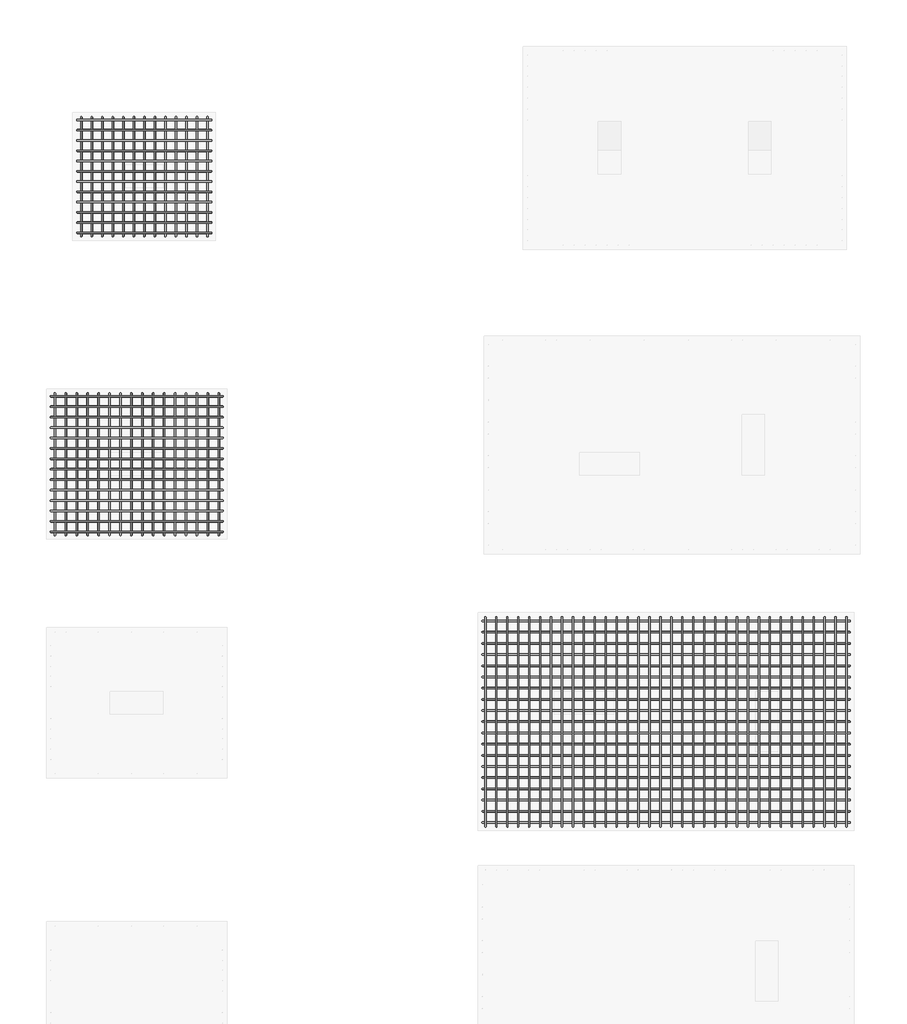
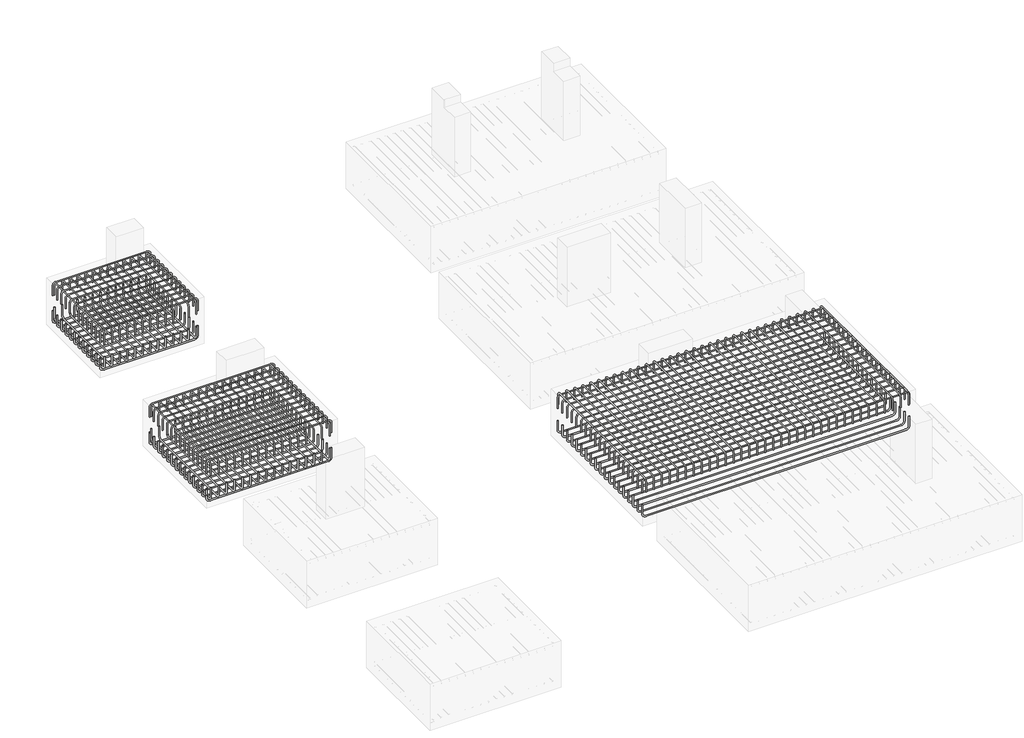
# One storey, part 11 of 21: 11 reinforcing bars.
"""IFC4 building model written with IfcOpenShell, lengths in millimetres."""

from ifc_helpers import new_model, si_unit, point, frame, origin, place, context, project, spatial, polyline, circle_curve, trimmed, segment, composite_curve, source, transform, mapped, element, save
from ifc_brep_helpers import swept_disk

model = new_model("IFC4")

# Units and contexts
model_context = context("Model", 3, world=origin())
ifc_project = project(units=[si_unit("LENGTHUNIT", "METRE", prefix="MILLI")], contexts=[model_context])

# Site, building, storey
site = spatial("IfcSite", under=ifc_project)
building = spatial("IfcBuilding", under=site)
storey = spatial("IfcBuildingStorey", under=building, Elevation=-1100.0)

# Reinforcing bars
placement = place(None, origin())
reinforcing_bar_shape = source(origin(), model_context, "Body", "SolidModel", [
    swept_disk(composite_curve([segment(polyline([(-23210.8326863, 15207.9216575, -1700.0), (-23210.8326863, 15207.9216575, -1882.5)]), True, "CONTINUOUS"), segment(trimmed(circle_curve(frame((-23268.3326863, 15207.9216575, -1882.5), z_axis=(0.0, 1.0, 0.0), x_axis=(57.5, 0.0, 0.0)), 57.5), [point((-23210.8326863, 15207.9216575, -1882.5))], [point((-23268.3326863, 15207.9216575, -1940.0))], True, "CARTESIAN"), True, "CONTINUOUS"), segment(polyline([(-23268.3326863, 15207.9216575, -1940.0), (-24933.3326863, 15207.9216575, -1940.0)]), True, "CONTINUOUS"), segment(trimmed(circle_curve(frame((-24933.3326863, 15207.9216575, -1882.5), z_axis=(0.0, 1.0, 0.0), x_axis=(0.0, 0.0, -57.5)), 57.5), [point((-24933.3326863, 15207.9216575, -1940.0))], [point((-24990.8326863, 15207.9216575, -1882.5))], True, "CARTESIAN"), True, "CONTINUOUS"), segment(polyline([(-24990.8326863, 15207.9216575, -1882.5), (-24990.8326863, 15207.9216575, -1700.0)]), True, "CONTINUOUS")], self_intersect=False), 10.0),
])
element("IfcReinforcingBar", 1, at=placement, inside=storey, context=model_context, shape_type="MappedRepresentation", body=[
    mapped(reinforcing_bar_shape, transform((0.0, 0.0, 0.0), x_axis=(1.0, 0.0, 0.0), y_axis=(0.0, 1.0, 0.0), z_axis=(0.0, 0.0, 1.0))),
    mapped(reinforcing_bar_shape, transform((0.0, -136.5188719, 0.0), x_axis=(1.0, 0.0, 0.0), y_axis=(0.0, 1.0, 0.0), z_axis=(0.0, 0.0, 1.0))),
    mapped(reinforcing_bar_shape, transform((0.0, -273.0377439, 0.0), x_axis=(1.0, 0.0, 0.0), y_axis=(0.0, 1.0, 0.0), z_axis=(0.0, 0.0, 1.0))),
    mapped(reinforcing_bar_shape, transform((0.0, -409.5566158, 0.0), x_axis=(1.0, 0.0, 0.0), y_axis=(0.0, 1.0, 0.0), z_axis=(0.0, 0.0, 1.0))),
    mapped(reinforcing_bar_shape, transform((0.0, -546.0754878, 0.0), x_axis=(1.0, 0.0, 0.0), y_axis=(0.0, 1.0, 0.0), z_axis=(0.0, 0.0, 1.0))),
    mapped(reinforcing_bar_shape, transform((0.0, -682.5943597, 0.0), x_axis=(1.0, 0.0, 0.0), y_axis=(0.0, 1.0, 0.0), z_axis=(0.0, 0.0, 1.0))),
    mapped(reinforcing_bar_shape, transform((0.0, -819.1132316, 0.0), x_axis=(1.0, 0.0, 0.0), y_axis=(0.0, 1.0, 0.0), z_axis=(0.0, 0.0, 1.0))),
    mapped(reinforcing_bar_shape, transform((0.0, -955.6321036, 0.0), x_axis=(1.0, 0.0, 0.0), y_axis=(0.0, 1.0, 0.0), z_axis=(0.0, 0.0, 1.0))),
    mapped(reinforcing_bar_shape, transform((0.0, -1092.1509755, 0.0), x_axis=(1.0, 0.0, 0.0), y_axis=(0.0, 1.0, 0.0), z_axis=(0.0, 0.0, 1.0))),
    mapped(reinforcing_bar_shape, transform((0.0, -1228.6698475, 0.0), x_axis=(1.0, 0.0, 0.0), y_axis=(0.0, 1.0, 0.0), z_axis=(0.0, 0.0, 1.0))),
    mapped(reinforcing_bar_shape, transform((0.0, -1365.1887194, 0.0), x_axis=(1.0, 0.0, 0.0), y_axis=(0.0, 1.0, 0.0), z_axis=(0.0, 0.0, 1.0))),
    mapped(reinforcing_bar_shape, transform((0.0, -1501.7075913, 0.0), x_axis=(1.0, 0.0, 0.0), y_axis=(0.0, 1.0, 0.0), z_axis=(0.0, 0.0, 1.0))),
])
reinforcing_bar_2_shape = source(origin(), model_context, "Body", "SolidModel", [
    swept_disk(composite_curve([segment(polyline([(-24992.8826863, 15207.9216575, -1400.0), (-24992.8826863, 15207.9216575, -1213.4)]), True, "CONTINUOUS"), segment(trimmed(circle_curve(frame((-24937.4326863, 15207.9216575, -1213.4), z_axis=(0.0, 1.0, 0.0), x_axis=(-55.45000000000073, 0.0, 0.0)), 55.45), [point((-24992.8826863, 15207.9216575, -1213.4))], [point((-24937.4326863, 15207.9216575, -1157.95))], True, "CARTESIAN"), True, "CONTINUOUS"), segment(polyline([(-24937.4326863, 15207.9216575, -1157.95), (-23264.2326863, 15207.9216575, -1157.95)]), True, "CONTINUOUS"), segment(trimmed(circle_curve(frame((-23264.2326863, 15207.9216575, -1213.4), z_axis=(0.0, 1.0, 0.0), x_axis=(0.0, 0.0, 55.450000000000045)), 55.45), [point((-23264.2326863, 15207.9216575, -1157.95))], [point((-23208.7826863, 15207.9216575, -1213.4))], True, "CARTESIAN"), True, "CONTINUOUS"), segment(polyline([(-23208.7826863, 15207.9216575, -1213.4), (-23208.7826863, 15207.9216575, -1400.0)]), True, "CONTINUOUS")], self_intersect=False), 7.95),
])
element("IfcReinforcingBar", 2, at=placement, inside=storey, context=model_context, shape_type="MappedRepresentation", body=[
    mapped(reinforcing_bar_2_shape, transform((0.0, 0.0, 0.0), x_axis=(1.0, 0.0, 0.0), y_axis=(0.0, 1.0, 0.0), z_axis=(0.0, 0.0, 1.0))),
    mapped(reinforcing_bar_2_shape, transform((0.0, -136.5188719, 0.0), x_axis=(1.0, 0.0, 0.0), y_axis=(0.0, 1.0, 0.0), z_axis=(0.0, 0.0, 1.0))),
    mapped(reinforcing_bar_2_shape, transform((0.0, -273.0377439, 0.0), x_axis=(1.0, 0.0, 0.0), y_axis=(0.0, 1.0, 0.0), z_axis=(0.0, 0.0, 1.0))),
    mapped(reinforcing_bar_2_shape, transform((0.0, -409.5566158, 0.0), x_axis=(1.0, 0.0, 0.0), y_axis=(0.0, 1.0, 0.0), z_axis=(0.0, 0.0, 1.0))),
    mapped(reinforcing_bar_2_shape, transform((0.0, -546.0754878, 0.0), x_axis=(1.0, 0.0, 0.0), y_axis=(0.0, 1.0, 0.0), z_axis=(0.0, 0.0, 1.0))),
    mapped(reinforcing_bar_2_shape, transform((0.0, -682.5943597, 0.0), x_axis=(1.0, 0.0, 0.0), y_axis=(0.0, 1.0, 0.0), z_axis=(0.0, 0.0, 1.0))),
    mapped(reinforcing_bar_2_shape, transform((0.0, -819.1132316, 0.0), x_axis=(1.0, 0.0, 0.0), y_axis=(0.0, 1.0, 0.0), z_axis=(0.0, 0.0, 1.0))),
    mapped(reinforcing_bar_2_shape, transform((0.0, -955.6321036, 0.0), x_axis=(1.0, 0.0, 0.0), y_axis=(0.0, 1.0, 0.0), z_axis=(0.0, 0.0, 1.0))),
    mapped(reinforcing_bar_2_shape, transform((0.0, -1092.1509755, 0.0), x_axis=(1.0, 0.0, 0.0), y_axis=(0.0, 1.0, 0.0), z_axis=(0.0, 0.0, 1.0))),
    mapped(reinforcing_bar_2_shape, transform((0.0, -1228.6698475, 0.0), x_axis=(1.0, 0.0, 0.0), y_axis=(0.0, 1.0, 0.0), z_axis=(0.0, 0.0, 1.0))),
    mapped(reinforcing_bar_2_shape, transform((0.0, -1365.1887194, 0.0), x_axis=(1.0, 0.0, 0.0), y_axis=(0.0, 1.0, 0.0), z_axis=(0.0, 0.0, 1.0))),
    mapped(reinforcing_bar_2_shape, transform((0.0, -1501.7075913, 0.0), x_axis=(1.0, 0.0, 0.0), y_axis=(0.0, 1.0, 0.0), z_axis=(0.0, 0.0, 1.0))),
])
reinforcing_bar_3_shape = source(origin(), model_context, "Body", "SolidModel", [
    swept_disk(composite_curve([segment(polyline([(-23260.6168504, 15246.2204288, -1428.1111113), (-23260.6168504, 15246.2204288, -1241.5111113)]), True, "CONTINUOUS"), segment(trimmed(circle_curve(frame((-23260.6168504, 15190.7704288, -1241.5111113), z_axis=(1.0, 0.0, 0.0), x_axis=(0.0, 55.44999999999891, 0.0)), 55.45), [point((-23260.6168504, 15246.2204288, -1241.5111113))], [point((-23260.6168504, 15190.7704288, -1186.0611113))], True, "CARTESIAN"), True, "CONTINUOUS"), segment(polyline([(-23260.6168504, 15190.7704288, -1186.0611113), (-23260.6168504, 13717.5704288, -1186.0611113)]), True, "CONTINUOUS"), segment(trimmed(circle_curve(frame((-23260.6168504, 13717.5704288, -1241.5111113), z_axis=(1.0, 0.0, 0.0), x_axis=(0.0, 0.0, 55.450000000000045)), 55.45), [point((-23260.6168504, 13717.5704288, -1186.0611113))], [point((-23260.6168504, 13662.1204288, -1241.5111113))], True, "CARTESIAN"), True, "CONTINUOUS"), segment(polyline([(-23260.6168504, 13662.1204288, -1241.5111113), (-23260.6168504, 13662.1204288, -1428.1111113)]), True, "CONTINUOUS")], self_intersect=False), 7.95),
])
element("IfcReinforcingBar", 3, at=placement, inside=storey, context=model_context, shape_type="MappedRepresentation", body=[
    mapped(reinforcing_bar_3_shape, transform((0.0, 0.0, 0.0), x_axis=(1.0, 0.0, 0.0), y_axis=(0.0, 1.0, 0.0), z_axis=(0.0, 0.0, 1.0))),
    mapped(reinforcing_bar_3_shape, transform((-139.8994495, 0.0, 0.0), x_axis=(1.0, 0.0, 0.0), y_axis=(0.0, 1.0, 0.0), z_axis=(0.0, 0.0, 1.0))),
    mapped(reinforcing_bar_3_shape, transform((-279.7988989, 0.0, 0.0), x_axis=(1.0, 0.0, 0.0), y_axis=(0.0, 1.0, 0.0), z_axis=(0.0, 0.0, 1.0))),
    mapped(reinforcing_bar_3_shape, transform((-419.6983484, 0.0, 0.0), x_axis=(1.0, 0.0, 0.0), y_axis=(0.0, 1.0, 0.0), z_axis=(0.0, 0.0, 1.0))),
    mapped(reinforcing_bar_3_shape, transform((-559.5977978, 0.0, 0.0), x_axis=(1.0, 0.0, 0.0), y_axis=(0.0, 1.0, 0.0), z_axis=(0.0, 0.0, 1.0))),
    mapped(reinforcing_bar_3_shape, transform((-699.4972473, 0.0, 0.0), x_axis=(1.0, 0.0, 0.0), y_axis=(0.0, 1.0, 0.0), z_axis=(0.0, 0.0, 1.0))),
    mapped(reinforcing_bar_3_shape, transform((-839.3966967, 0.0, 0.0), x_axis=(1.0, 0.0, 0.0), y_axis=(0.0, 1.0, 0.0), z_axis=(0.0, 0.0, 1.0))),
    mapped(reinforcing_bar_3_shape, transform((-979.2961462, 0.0, 0.0), x_axis=(1.0, 0.0, 0.0), y_axis=(0.0, 1.0, 0.0), z_axis=(0.0, 0.0, 1.0))),
    mapped(reinforcing_bar_3_shape, transform((-1119.1955956, 0.0, 0.0), x_axis=(1.0, 0.0, 0.0), y_axis=(0.0, 1.0, 0.0), z_axis=(0.0, 0.0, 1.0))),
    mapped(reinforcing_bar_3_shape, transform((-1259.0950451, 0.0, 0.0), x_axis=(1.0, 0.0, 0.0), y_axis=(0.0, 1.0, 0.0), z_axis=(0.0, 0.0, 1.0))),
    mapped(reinforcing_bar_3_shape, transform((-1398.9944945, 0.0, 0.0), x_axis=(1.0, 0.0, 0.0), y_axis=(0.0, 1.0, 0.0), z_axis=(0.0, 0.0, 1.0))),
    mapped(reinforcing_bar_3_shape, transform((-1538.893944, 0.0, 0.0), x_axis=(1.0, 0.0, 0.0), y_axis=(0.0, 1.0, 0.0), z_axis=(0.0, 0.0, 1.0))),
    mapped(reinforcing_bar_3_shape, transform((-1678.7933934, 0.0, 0.0), x_axis=(1.0, 0.0, 0.0), y_axis=(0.0, 1.0, 0.0), z_axis=(0.0, 0.0, 1.0))),
])
reinforcing_bar_4_shape = source(origin(), model_context, "Body", "SolidModel", [
    swept_disk(composite_curve([segment(polyline([(-24939.4102438, 15244.1704288, -1669.8442859), (-24939.4102438, 15244.1704288, -1852.3442859)]), True, "CONTINUOUS"), segment(trimmed(circle_curve(frame((-24939.4102438, 15186.6704288, -1852.3442859), z_axis=(-1.0, 0.0, 0.0), x_axis=(0.0, 57.5, 0.0)), 57.5), [point((-24939.4102438, 15244.1704288, -1852.3442859))], [point((-24939.4102438, 15186.6704288, -1909.8442859))], True, "CARTESIAN"), True, "CONTINUOUS"), segment(polyline([(-24939.4102438, 15186.6704288, -1909.8442859), (-24939.4102438, 13721.6704288, -1909.8442859)]), True, "CONTINUOUS"), segment(trimmed(circle_curve(frame((-24939.4102438, 13721.6704288, -1852.3442859), z_axis=(-1.0, 0.0, 0.0), x_axis=(0.0, 0.0, -57.5)), 57.5), [point((-24939.4102438, 13721.6704288, -1909.8442859))], [point((-24939.4102438, 13664.1704288, -1852.3442859))], True, "CARTESIAN"), True, "CONTINUOUS"), segment(polyline([(-24939.4102438, 13664.1704288, -1852.3442859), (-24939.4102438, 13664.1704288, -1669.8442859)]), True, "CONTINUOUS")], self_intersect=False), 10.0),
])
element("IfcReinforcingBar", 4, at=placement, inside=storey, context=model_context, shape_type="MappedRepresentation", body=[
    mapped(reinforcing_bar_4_shape, transform((0.0, 0.0, 0.0), x_axis=(1.0, 0.0, 0.0), y_axis=(0.0, 1.0, 0.0), z_axis=(0.0, 0.0, 1.0))),
    mapped(reinforcing_bar_4_shape, transform((139.8994495, 0.0, 0.0), x_axis=(1.0, 0.0, 0.0), y_axis=(0.0, 1.0, 0.0), z_axis=(0.0, 0.0, 1.0))),
    mapped(reinforcing_bar_4_shape, transform((279.7988989, 0.0, 0.0), x_axis=(1.0, 0.0, 0.0), y_axis=(0.0, 1.0, 0.0), z_axis=(0.0, 0.0, 1.0))),
    mapped(reinforcing_bar_4_shape, transform((419.6983484, 0.0, 0.0), x_axis=(1.0, 0.0, 0.0), y_axis=(0.0, 1.0, 0.0), z_axis=(0.0, 0.0, 1.0))),
    mapped(reinforcing_bar_4_shape, transform((559.5977978, 0.0, 0.0), x_axis=(1.0, 0.0, 0.0), y_axis=(0.0, 1.0, 0.0), z_axis=(0.0, 0.0, 1.0))),
    mapped(reinforcing_bar_4_shape, transform((699.4972473, 0.0, 0.0), x_axis=(1.0, 0.0, 0.0), y_axis=(0.0, 1.0, 0.0), z_axis=(0.0, 0.0, 1.0))),
    mapped(reinforcing_bar_4_shape, transform((839.3966967, 0.0, 0.0), x_axis=(1.0, 0.0, 0.0), y_axis=(0.0, 1.0, 0.0), z_axis=(0.0, 0.0, 1.0))),
    mapped(reinforcing_bar_4_shape, transform((979.2961462, 0.0, 0.0), x_axis=(1.0, 0.0, 0.0), y_axis=(0.0, 1.0, 0.0), z_axis=(0.0, 0.0, 1.0))),
    mapped(reinforcing_bar_4_shape, transform((1119.1955956, 0.0, 0.0), x_axis=(1.0, 0.0, 0.0), y_axis=(0.0, 1.0, 0.0), z_axis=(0.0, 0.0, 1.0))),
    mapped(reinforcing_bar_4_shape, transform((1259.0950451, 0.0, 0.0), x_axis=(1.0, 0.0, 0.0), y_axis=(0.0, 1.0, 0.0), z_axis=(0.0, 0.0, 1.0))),
    mapped(reinforcing_bar_4_shape, transform((1398.9944945, 0.0, 0.0), x_axis=(1.0, 0.0, 0.0), y_axis=(0.0, 1.0, 0.0), z_axis=(0.0, 0.0, 1.0))),
    mapped(reinforcing_bar_4_shape, transform((1538.893944, 0.0, 0.0), x_axis=(1.0, 0.0, 0.0), y_axis=(0.0, 1.0, 0.0), z_axis=(0.0, 0.0, 1.0))),
    mapped(reinforcing_bar_4_shape, transform((1678.7933934, 0.0, 0.0), x_axis=(1.0, 0.0, 0.0), y_axis=(0.0, 1.0, 0.0), z_axis=(0.0, 0.0, 1.0))),
])
reinforcing_bar_5_shape = source(origin(), model_context, "Body", "SolidModel", [
    swept_disk(composite_curve([segment(polyline([(-23061.1351198, 11532.9767109, -1700.0), (-23061.1351198, 11532.9767109, -1882.5)]), True, "CONTINUOUS"), segment(trimmed(circle_curve(frame((-23118.6351198, 11532.9767109, -1882.5), z_axis=(0.0, 1.0, 0.0), x_axis=(57.5, 0.0, 0.0)), 57.5), [point((-23061.1351198, 11532.9767109, -1882.5))], [point((-23118.6351198, 11532.9767109, -1940.0))], True, "CARTESIAN"), True, "CONTINUOUS"), segment(polyline([(-23118.6351198, 11532.9767109, -1940.0), (-25283.6351198, 11532.9767109, -1940.0)]), True, "CONTINUOUS"), segment(trimmed(circle_curve(frame((-25283.6351198, 11532.9767109, -1882.5), z_axis=(0.0, 1.0, 0.0), x_axis=(0.0, 0.0, -57.5)), 57.5), [point((-25283.6351198, 11532.9767109, -1940.0))], [point((-25341.1351198, 11532.9767109, -1882.5))], True, "CARTESIAN"), True, "CONTINUOUS"), segment(polyline([(-25341.1351198, 11532.9767109, -1882.5), (-25341.1351198, 11532.9767109, -1700.0)]), True, "CONTINUOUS")], self_intersect=False), 10.0),
])
element("IfcReinforcingBar", 5, at=placement, inside=storey, context=model_context, shape_type="MappedRepresentation", body=[
    mapped(reinforcing_bar_5_shape, transform((0.0, 0.0, 0.0), x_axis=(1.0, 0.0, 0.0), y_axis=(0.0, 1.0, 0.0), z_axis=(0.0, 0.0, 1.0))),
    mapped(reinforcing_bar_5_shape, transform((0.0, -138.5928916, 0.0), x_axis=(1.0, 0.0, 0.0), y_axis=(0.0, 1.0, 0.0), z_axis=(0.0, 0.0, 1.0))),
    mapped(reinforcing_bar_5_shape, transform((0.0, -277.1857833, 0.0), x_axis=(1.0, 0.0, 0.0), y_axis=(0.0, 1.0, 0.0), z_axis=(0.0, 0.0, 1.0))),
    mapped(reinforcing_bar_5_shape, transform((0.0, -415.7786749, 0.0), x_axis=(1.0, 0.0, 0.0), y_axis=(0.0, 1.0, 0.0), z_axis=(0.0, 0.0, 1.0))),
    mapped(reinforcing_bar_5_shape, transform((0.0, -554.3715666, 0.0), x_axis=(1.0, 0.0, 0.0), y_axis=(0.0, 1.0, 0.0), z_axis=(0.0, 0.0, 1.0))),
    mapped(reinforcing_bar_5_shape, transform((0.0, -692.9644582, 0.0), x_axis=(1.0, 0.0, 0.0), y_axis=(0.0, 1.0, 0.0), z_axis=(0.0, 0.0, 1.0))),
    mapped(reinforcing_bar_5_shape, transform((0.0, -831.5573499, 0.0), x_axis=(1.0, 0.0, 0.0), y_axis=(0.0, 1.0, 0.0), z_axis=(0.0, 0.0, 1.0))),
    mapped(reinforcing_bar_5_shape, transform((0.0, -970.1502415, 0.0), x_axis=(1.0, 0.0, 0.0), y_axis=(0.0, 1.0, 0.0), z_axis=(0.0, 0.0, 1.0))),
    mapped(reinforcing_bar_5_shape, transform((0.0, -1108.7431331, 0.0), x_axis=(1.0, 0.0, 0.0), y_axis=(0.0, 1.0, 0.0), z_axis=(0.0, 0.0, 1.0))),
    mapped(reinforcing_bar_5_shape, transform((0.0, -1247.3360248, 0.0), x_axis=(1.0, 0.0, 0.0), y_axis=(0.0, 1.0, 0.0), z_axis=(0.0, 0.0, 1.0))),
    mapped(reinforcing_bar_5_shape, transform((0.0, -1385.9289164, 0.0), x_axis=(1.0, 0.0, 0.0), y_axis=(0.0, 1.0, 0.0), z_axis=(0.0, 0.0, 1.0))),
    mapped(reinforcing_bar_5_shape, transform((0.0, -1524.5218081, 0.0), x_axis=(1.0, 0.0, 0.0), y_axis=(0.0, 1.0, 0.0), z_axis=(0.0, 0.0, 1.0))),
    mapped(reinforcing_bar_5_shape, transform((0.0, -1663.1146997, 0.0), x_axis=(1.0, 0.0, 0.0), y_axis=(0.0, 1.0, 0.0), z_axis=(0.0, 0.0, 1.0))),
    mapped(reinforcing_bar_5_shape, transform((0.0, -1801.7075913, 0.0), x_axis=(1.0, 0.0, 0.0), y_axis=(0.0, 1.0, 0.0), z_axis=(0.0, 0.0, 1.0))),
])
reinforcing_bar_6_shape = source(origin(), model_context, "Body", "SolidModel", [
    swept_disk(composite_curve([segment(polyline([(-25343.1851198, 11532.9767109, -1400.0), (-25343.1851198, 11532.9767109, -1213.4)]), True, "CONTINUOUS"), segment(trimmed(circle_curve(frame((-25287.7351198, 11532.9767109, -1213.4), z_axis=(0.0, 1.0, 0.0), x_axis=(-55.45000000000073, 0.0, 0.0)), 55.45), [point((-25343.1851198, 11532.9767109, -1213.4))], [point((-25287.7351198, 11532.9767109, -1157.95))], True, "CARTESIAN"), True, "CONTINUOUS"), segment(polyline([(-25287.7351198, 11532.9767109, -1157.95), (-23114.5351198, 11532.9767109, -1157.95)]), True, "CONTINUOUS"), segment(trimmed(circle_curve(frame((-23114.5351198, 11532.9767109, -1213.4), z_axis=(0.0, 1.0, 0.0), x_axis=(0.0, 0.0, 55.450000000000045)), 55.45), [point((-23114.5351198, 11532.9767109, -1157.95))], [point((-23059.0851198, 11532.9767109, -1213.4))], True, "CARTESIAN"), True, "CONTINUOUS"), segment(polyline([(-23059.0851198, 11532.9767109, -1213.4), (-23059.0851198, 11532.9767109, -1400.0)]), True, "CONTINUOUS")], self_intersect=False), 7.95),
])
element("IfcReinforcingBar", 6, at=placement, inside=storey, context=model_context, shape_type="MappedRepresentation", body=[
    mapped(reinforcing_bar_6_shape, transform((0.0, 0.0, 0.0), x_axis=(1.0, 0.0, 0.0), y_axis=(0.0, 1.0, 0.0), z_axis=(0.0, 0.0, 1.0))),
    mapped(reinforcing_bar_6_shape, transform((0.0, -138.5928916, 0.0), x_axis=(1.0, 0.0, 0.0), y_axis=(0.0, 1.0, 0.0), z_axis=(0.0, 0.0, 1.0))),
    mapped(reinforcing_bar_6_shape, transform((0.0, -277.1857833, 0.0), x_axis=(1.0, 0.0, 0.0), y_axis=(0.0, 1.0, 0.0), z_axis=(0.0, 0.0, 1.0))),
    mapped(reinforcing_bar_6_shape, transform((0.0, -415.7786749, 0.0), x_axis=(1.0, 0.0, 0.0), y_axis=(0.0, 1.0, 0.0), z_axis=(0.0, 0.0, 1.0))),
    mapped(reinforcing_bar_6_shape, transform((0.0, -554.3715666, 0.0), x_axis=(1.0, 0.0, 0.0), y_axis=(0.0, 1.0, 0.0), z_axis=(0.0, 0.0, 1.0))),
    mapped(reinforcing_bar_6_shape, transform((0.0, -692.9644582, 0.0), x_axis=(1.0, 0.0, 0.0), y_axis=(0.0, 1.0, 0.0), z_axis=(0.0, 0.0, 1.0))),
    mapped(reinforcing_bar_6_shape, transform((0.0, -831.5573499, 0.0), x_axis=(1.0, 0.0, 0.0), y_axis=(0.0, 1.0, 0.0), z_axis=(0.0, 0.0, 1.0))),
    mapped(reinforcing_bar_6_shape, transform((0.0, -970.1502415, 0.0), x_axis=(1.0, 0.0, 0.0), y_axis=(0.0, 1.0, 0.0), z_axis=(0.0, 0.0, 1.0))),
    mapped(reinforcing_bar_6_shape, transform((0.0, -1108.7431331, 0.0), x_axis=(1.0, 0.0, 0.0), y_axis=(0.0, 1.0, 0.0), z_axis=(0.0, 0.0, 1.0))),
    mapped(reinforcing_bar_6_shape, transform((0.0, -1247.3360248, 0.0), x_axis=(1.0, 0.0, 0.0), y_axis=(0.0, 1.0, 0.0), z_axis=(0.0, 0.0, 1.0))),
    mapped(reinforcing_bar_6_shape, transform((0.0, -1385.9289164, 0.0), x_axis=(1.0, 0.0, 0.0), y_axis=(0.0, 1.0, 0.0), z_axis=(0.0, 0.0, 1.0))),
    mapped(reinforcing_bar_6_shape, transform((0.0, -1524.5218081, 0.0), x_axis=(1.0, 0.0, 0.0), y_axis=(0.0, 1.0, 0.0), z_axis=(0.0, 0.0, 1.0))),
    mapped(reinforcing_bar_6_shape, transform((0.0, -1663.1146997, 0.0), x_axis=(1.0, 0.0, 0.0), y_axis=(0.0, 1.0, 0.0), z_axis=(0.0, 0.0, 1.0))),
    mapped(reinforcing_bar_6_shape, transform((0.0, -1801.7075913, 0.0), x_axis=(1.0, 0.0, 0.0), y_axis=(0.0, 1.0, 0.0), z_axis=(0.0, 0.0, 1.0))),
])
reinforcing_bar_7_shape = source(origin(), model_context, "Body", "SolidModel", [
    swept_disk(composite_curve([segment(polyline([(-23110.9192838, 11571.2754822, -1428.1111113), (-23110.9192838, 11571.2754822, -1241.5111113)]), True, "CONTINUOUS"), segment(trimmed(circle_curve(frame((-23110.9192838, 11515.8254822, -1241.5111113), z_axis=(1.0, 0.0, 0.0), x_axis=(0.0, 55.45000000000073, 0.0)), 55.45), [point((-23110.9192838, 11571.2754822, -1241.5111113))], [point((-23110.9192838, 11515.8254822, -1186.0611113))], True, "CARTESIAN"), True, "CONTINUOUS"), segment(polyline([(-23110.9192838, 11515.8254822, -1186.0611113), (-23110.9192838, 9742.6254822, -1186.0611113)]), True, "CONTINUOUS"), segment(trimmed(circle_curve(frame((-23110.9192838, 9742.6254822, -1241.5111113), z_axis=(1.0, 0.0, 0.0), x_axis=(0.0, 0.0, 55.450000000000045)), 55.45), [point((-23110.9192838, 9742.6254822, -1186.0611113))], [point((-23110.9192838, 9687.1754822, -1241.5111113))], True, "CARTESIAN"), True, "CONTINUOUS"), segment(polyline([(-23110.9192838, 9687.1754822, -1241.5111113), (-23110.9192838, 9687.1754822, -1428.1111113)]), True, "CONTINUOUS")], self_intersect=False), 7.95),
])
element("IfcReinforcingBar", 7, at=placement, inside=storey, context=model_context, shape_type="MappedRepresentation", body=[
    mapped(reinforcing_bar_7_shape, transform((0.0, 0.0, 0.0), x_axis=(1.0, 0.0, 0.0), y_axis=(0.0, 1.0, 0.0), z_axis=(0.0, 0.0, 1.0))),
    mapped(reinforcing_bar_7_shape, transform((-145.2528929, 0.0, 0.0), x_axis=(1.0, 0.0, 0.0), y_axis=(0.0, 1.0, 0.0), z_axis=(0.0, 0.0, 1.0))),
    mapped(reinforcing_bar_7_shape, transform((-290.5057858, 0.0, 0.0), x_axis=(1.0, 0.0, 0.0), y_axis=(0.0, 1.0, 0.0), z_axis=(0.0, 0.0, 1.0))),
    mapped(reinforcing_bar_7_shape, transform((-435.7586787, 0.0, 0.0), x_axis=(1.0, 0.0, 0.0), y_axis=(0.0, 1.0, 0.0), z_axis=(0.0, 0.0, 1.0))),
    mapped(reinforcing_bar_7_shape, transform((-581.0115716, 0.0, 0.0), x_axis=(1.0, 0.0, 0.0), y_axis=(0.0, 1.0, 0.0), z_axis=(0.0, 0.0, 1.0))),
    mapped(reinforcing_bar_7_shape, transform((-726.2644645, 0.0, 0.0), x_axis=(1.0, 0.0, 0.0), y_axis=(0.0, 1.0, 0.0), z_axis=(0.0, 0.0, 1.0))),
    mapped(reinforcing_bar_7_shape, transform((-871.5173574, 0.0, 0.0), x_axis=(1.0, 0.0, 0.0), y_axis=(0.0, 1.0, 0.0), z_axis=(0.0, 0.0, 1.0))),
    mapped(reinforcing_bar_7_shape, transform((-1016.7702503, 0.0, 0.0), x_axis=(1.0, 0.0, 0.0), y_axis=(0.0, 1.0, 0.0), z_axis=(0.0, 0.0, 1.0))),
    mapped(reinforcing_bar_7_shape, transform((-1162.0231432, 0.0, 0.0), x_axis=(1.0, 0.0, 0.0), y_axis=(0.0, 1.0, 0.0), z_axis=(0.0, 0.0, 1.0))),
    mapped(reinforcing_bar_7_shape, transform((-1307.276036, 0.0, 0.0), x_axis=(1.0, 0.0, 0.0), y_axis=(0.0, 1.0, 0.0), z_axis=(0.0, 0.0, 1.0))),
    mapped(reinforcing_bar_7_shape, transform((-1452.5289289, 0.0, 0.0), x_axis=(1.0, 0.0, 0.0), y_axis=(0.0, 1.0, 0.0), z_axis=(0.0, 0.0, 1.0))),
    mapped(reinforcing_bar_7_shape, transform((-1597.7818218, 0.0, 0.0), x_axis=(1.0, 0.0, 0.0), y_axis=(0.0, 1.0, 0.0), z_axis=(0.0, 0.0, 1.0))),
    mapped(reinforcing_bar_7_shape, transform((-1743.0347147, 0.0, 0.0), x_axis=(1.0, 0.0, 0.0), y_axis=(0.0, 1.0, 0.0), z_axis=(0.0, 0.0, 1.0))),
    mapped(reinforcing_bar_7_shape, transform((-1888.2876076, 0.0, 0.0), x_axis=(1.0, 0.0, 0.0), y_axis=(0.0, 1.0, 0.0), z_axis=(0.0, 0.0, 1.0))),
    mapped(reinforcing_bar_7_shape, transform((-2033.5405005, 0.0, 0.0), x_axis=(1.0, 0.0, 0.0), y_axis=(0.0, 1.0, 0.0), z_axis=(0.0, 0.0, 1.0))),
    mapped(reinforcing_bar_7_shape, transform((-2178.7933934, 0.0, 0.0), x_axis=(1.0, 0.0, 0.0), y_axis=(0.0, 1.0, 0.0), z_axis=(0.0, 0.0, 1.0))),
])
reinforcing_bar_8_shape = source(origin(), model_context, "Body", "SolidModel", [
    swept_disk(composite_curve([segment(polyline([(-25289.7126772, 11569.2254822, -1669.8442859), (-25289.7126772, 11569.2254822, -1852.3442859)]), True, "CONTINUOUS"), segment(trimmed(circle_curve(frame((-25289.7126772, 11511.7254822, -1852.3442859), z_axis=(-1.0, 0.0, 0.0), x_axis=(0.0, 57.5, 0.0)), 57.5), [point((-25289.7126772, 11569.2254822, -1852.3442859))], [point((-25289.7126772, 11511.7254822, -1909.8442859))], True, "CARTESIAN"), True, "CONTINUOUS"), segment(polyline([(-25289.7126772, 11511.7254822, -1909.8442859), (-25289.7126772, 9746.7254822, -1909.8442859)]), True, "CONTINUOUS"), segment(trimmed(circle_curve(frame((-25289.7126772, 9746.7254822, -1852.3442859), z_axis=(-1.0, 0.0, 0.0), x_axis=(0.0, 0.0, -57.5)), 57.5), [point((-25289.7126772, 9746.7254822, -1909.8442859))], [point((-25289.7126772, 9689.2254822, -1852.3442859))], True, "CARTESIAN"), True, "CONTINUOUS"), segment(polyline([(-25289.7126772, 9689.2254822, -1852.3442859), (-25289.7126772, 9689.2254822, -1669.8442859)]), True, "CONTINUOUS")], self_intersect=False), 10.0),
])
element("IfcReinforcingBar", 8, at=placement, inside=storey, context=model_context, shape_type="MappedRepresentation", body=[
    mapped(reinforcing_bar_8_shape, transform((0.0, 0.0, 0.0), x_axis=(1.0, 0.0, 0.0), y_axis=(0.0, 1.0, 0.0), z_axis=(0.0, 0.0, 1.0))),
    mapped(reinforcing_bar_8_shape, transform((145.2528929, 0.0, 0.0), x_axis=(1.0, 0.0, 0.0), y_axis=(0.0, 1.0, 0.0), z_axis=(0.0, 0.0, 1.0))),
    mapped(reinforcing_bar_8_shape, transform((290.5057858, 0.0, 0.0), x_axis=(1.0, 0.0, 0.0), y_axis=(0.0, 1.0, 0.0), z_axis=(0.0, 0.0, 1.0))),
    mapped(reinforcing_bar_8_shape, transform((435.7586787, 0.0, 0.0), x_axis=(1.0, 0.0, 0.0), y_axis=(0.0, 1.0, 0.0), z_axis=(0.0, 0.0, 1.0))),
    mapped(reinforcing_bar_8_shape, transform((581.0115716, 0.0, 0.0), x_axis=(1.0, 0.0, 0.0), y_axis=(0.0, 1.0, 0.0), z_axis=(0.0, 0.0, 1.0))),
    mapped(reinforcing_bar_8_shape, transform((726.2644645, 0.0, 0.0), x_axis=(1.0, 0.0, 0.0), y_axis=(0.0, 1.0, 0.0), z_axis=(0.0, 0.0, 1.0))),
    mapped(reinforcing_bar_8_shape, transform((871.5173574, 0.0, 0.0), x_axis=(1.0, 0.0, 0.0), y_axis=(0.0, 1.0, 0.0), z_axis=(0.0, 0.0, 1.0))),
    mapped(reinforcing_bar_8_shape, transform((1016.7702503, 0.0, 0.0), x_axis=(1.0, 0.0, 0.0), y_axis=(0.0, 1.0, 0.0), z_axis=(0.0, 0.0, 1.0))),
    mapped(reinforcing_bar_8_shape, transform((1162.0231432, 0.0, 0.0), x_axis=(1.0, 0.0, 0.0), y_axis=(0.0, 1.0, 0.0), z_axis=(0.0, 0.0, 1.0))),
    mapped(reinforcing_bar_8_shape, transform((1307.276036, 0.0, 0.0), x_axis=(1.0, 0.0, 0.0), y_axis=(0.0, 1.0, 0.0), z_axis=(0.0, 0.0, 1.0))),
    mapped(reinforcing_bar_8_shape, transform((1452.5289289, 0.0, 0.0), x_axis=(1.0, 0.0, 0.0), y_axis=(0.0, 1.0, 0.0), z_axis=(0.0, 0.0, 1.0))),
    mapped(reinforcing_bar_8_shape, transform((1597.7818218, 0.0, 0.0), x_axis=(1.0, 0.0, 0.0), y_axis=(0.0, 1.0, 0.0), z_axis=(0.0, 0.0, 1.0))),
    mapped(reinforcing_bar_8_shape, transform((1743.0347147, 0.0, 0.0), x_axis=(1.0, 0.0, 0.0), y_axis=(0.0, 1.0, 0.0), z_axis=(0.0, 0.0, 1.0))),
    mapped(reinforcing_bar_8_shape, transform((1888.2876076, 0.0, 0.0), x_axis=(1.0, 0.0, 0.0), y_axis=(0.0, 1.0, 0.0), z_axis=(0.0, 0.0, 1.0))),
    mapped(reinforcing_bar_8_shape, transform((2033.5405005, 0.0, 0.0), x_axis=(1.0, 0.0, 0.0), y_axis=(0.0, 1.0, 0.0), z_axis=(0.0, 0.0, 1.0))),
    mapped(reinforcing_bar_8_shape, transform((2178.7933934, 0.0, 0.0), x_axis=(1.0, 0.0, 0.0), y_axis=(0.0, 1.0, 0.0), z_axis=(0.0, 0.0, 1.0))),
])
reinforcing_bar_9_shape = source(origin(), model_context, "Body", "SolidModel", [
    swept_disk(composite_curve([segment(polyline([(-19564.5839151, 5812.1204288, -1400.0), (-19564.5839151, 5812.1204288, -1213.4)]), True, "CONTINUOUS"), segment(trimmed(circle_curve(frame((-19564.5839151, 5867.5704288, -1213.4), z_axis=(-1.0, 0.0, 0.0), x_axis=(0.0, -55.44999999999982, 0.0)), 55.45), [point((-19564.5839151, 5812.1204288, -1213.4))], [point((-19564.5839151, 5867.5704288, -1157.95))], True, "CARTESIAN"), True, "CONTINUOUS"), segment(polyline([(-19564.5839151, 5867.5704288, -1157.95), (-19564.5839151, 8540.7704288, -1157.95)]), True, "CONTINUOUS"), segment(trimmed(circle_curve(frame((-19564.5839151, 8540.7704288, -1213.4), z_axis=(-1.0, 0.0, 0.0), x_axis=(0.0, 0.0, 55.450000000000045)), 55.45), [point((-19564.5839151, 8540.7704288, -1157.95))], [point((-19564.5839151, 8596.2204288, -1213.4))], True, "CARTESIAN"), True, "CONTINUOUS"), segment(polyline([(-19564.5839151, 8596.2204288, -1213.4), (-19564.5839151, 8596.2204288, -1400.0)]), True, "CONTINUOUS")], self_intersect=False), 7.95),
])
element("IfcReinforcingBar", 9, at=placement, inside=storey, context=model_context, shape_type="MappedRepresentation", body=[
    mapped(reinforcing_bar_9_shape, transform((0.0, 0.0, 0.0), x_axis=(1.0, 0.0, 0.0), y_axis=(0.0, 1.0, 0.0), z_axis=(0.0, 0.0, 1.0))),
    mapped(reinforcing_bar_9_shape, transform((145.5062906, 0.0, 0.0), x_axis=(1.0, 0.0, 0.0), y_axis=(0.0, 1.0, 0.0), z_axis=(0.0, 0.0, 1.0))),
    mapped(reinforcing_bar_9_shape, transform((291.0125813, 0.0, 0.0), x_axis=(1.0, 0.0, 0.0), y_axis=(0.0, 1.0, 0.0), z_axis=(0.0, 0.0, 1.0))),
    mapped(reinforcing_bar_9_shape, transform((436.5188719, 0.0, 0.0), x_axis=(1.0, 0.0, 0.0), y_axis=(0.0, 1.0, 0.0), z_axis=(0.0, 0.0, 1.0))),
    mapped(reinforcing_bar_9_shape, transform((582.0251626, 0.0, 0.0), x_axis=(1.0, 0.0, 0.0), y_axis=(0.0, 1.0, 0.0), z_axis=(0.0, 0.0, 1.0))),
    mapped(reinforcing_bar_9_shape, transform((727.5314532, 0.0, 0.0), x_axis=(1.0, 0.0, 0.0), y_axis=(0.0, 1.0, 0.0), z_axis=(0.0, 0.0, 1.0))),
    mapped(reinforcing_bar_9_shape, transform((873.0377439, 0.0, 0.0), x_axis=(1.0, 0.0, 0.0), y_axis=(0.0, 1.0, 0.0), z_axis=(0.0, 0.0, 1.0))),
    mapped(reinforcing_bar_9_shape, transform((1018.5440345, 0.0, 0.0), x_axis=(1.0, 0.0, 0.0), y_axis=(0.0, 1.0, 0.0), z_axis=(0.0, 0.0, 1.0))),
    mapped(reinforcing_bar_9_shape, transform((1164.0503252, 0.0, 0.0), x_axis=(1.0, 0.0, 0.0), y_axis=(0.0, 1.0, 0.0), z_axis=(0.0, 0.0, 1.0))),
    mapped(reinforcing_bar_9_shape, transform((1309.5566158, 0.0, 0.0), x_axis=(1.0, 0.0, 0.0), y_axis=(0.0, 1.0, 0.0), z_axis=(0.0, 0.0, 1.0))),
    mapped(reinforcing_bar_9_shape, transform((1455.0629065, 0.0, 0.0), x_axis=(1.0, 0.0, 0.0), y_axis=(0.0, 1.0, 0.0), z_axis=(0.0, 0.0, 1.0))),
    mapped(reinforcing_bar_9_shape, transform((1600.5691971, 0.0, 0.0), x_axis=(1.0, 0.0, 0.0), y_axis=(0.0, 1.0, 0.0), z_axis=(0.0, 0.0, 1.0))),
    mapped(reinforcing_bar_9_shape, transform((1746.0754878, 0.0, 0.0), x_axis=(1.0, 0.0, 0.0), y_axis=(0.0, 1.0, 0.0), z_axis=(0.0, 0.0, 1.0))),
    mapped(reinforcing_bar_9_shape, transform((1891.5817784, 0.0, 0.0), x_axis=(1.0, 0.0, 0.0), y_axis=(0.0, 1.0, 0.0), z_axis=(0.0, 0.0, 1.0))),
    mapped(reinforcing_bar_9_shape, transform((2037.0880691, 0.0, 0.0), x_axis=(1.0, 0.0, 0.0), y_axis=(0.0, 1.0, 0.0), z_axis=(0.0, 0.0, 1.0))),
    mapped(reinforcing_bar_9_shape, transform((2182.5943597, 0.0, 0.0), x_axis=(1.0, 0.0, 0.0), y_axis=(0.0, 1.0, 0.0), z_axis=(0.0, 0.0, 1.0))),
    mapped(reinforcing_bar_9_shape, transform((2328.1006504, 0.0, 0.0), x_axis=(1.0, 0.0, 0.0), y_axis=(0.0, 1.0, 0.0), z_axis=(0.0, 0.0, 1.0))),
    mapped(reinforcing_bar_9_shape, transform((2473.606941, 0.0, 0.0), x_axis=(1.0, 0.0, 0.0), y_axis=(0.0, 1.0, 0.0), z_axis=(0.0, 0.0, 1.0))),
    mapped(reinforcing_bar_9_shape, transform((2619.1132316, 0.0, 0.0), x_axis=(1.0, 0.0, 0.0), y_axis=(0.0, 1.0, 0.0), z_axis=(0.0, 0.0, 1.0))),
    mapped(reinforcing_bar_9_shape, transform((2764.6195223, 0.0, 0.0), x_axis=(1.0, 0.0, 0.0), y_axis=(0.0, 1.0, 0.0), z_axis=(0.0, 0.0, 1.0))),
    mapped(reinforcing_bar_9_shape, transform((2910.1258129, 0.0, 0.0), x_axis=(1.0, 0.0, 0.0), y_axis=(0.0, 1.0, 0.0), z_axis=(0.0, 0.0, 1.0))),
    mapped(reinforcing_bar_9_shape, transform((3055.6321036, 0.0, 0.0), x_axis=(1.0, 0.0, 0.0), y_axis=(0.0, 1.0, 0.0), z_axis=(0.0, 0.0, 1.0))),
    mapped(reinforcing_bar_9_shape, transform((3201.1383942, 0.0, 0.0), x_axis=(1.0, 0.0, 0.0), y_axis=(0.0, 1.0, 0.0), z_axis=(0.0, 0.0, 1.0))),
    mapped(reinforcing_bar_9_shape, transform((3346.6446849, 0.0, 0.0), x_axis=(1.0, 0.0, 0.0), y_axis=(0.0, 1.0, 0.0), z_axis=(0.0, 0.0, 1.0))),
    mapped(reinforcing_bar_9_shape, transform((3492.1509755, 0.0, 0.0), x_axis=(1.0, 0.0, 0.0), y_axis=(0.0, 1.0, 0.0), z_axis=(0.0, 0.0, 1.0))),
    mapped(reinforcing_bar_9_shape, transform((3637.6572662, 0.0, 0.0), x_axis=(1.0, 0.0, 0.0), y_axis=(0.0, 1.0, 0.0), z_axis=(0.0, 0.0, 1.0))),
    mapped(reinforcing_bar_9_shape, transform((3783.1635568, 0.0, 0.0), x_axis=(1.0, 0.0, 0.0), y_axis=(0.0, 1.0, 0.0), z_axis=(0.0, 0.0, 1.0))),
    mapped(reinforcing_bar_9_shape, transform((3928.6698475, 0.0, 0.0), x_axis=(1.0, 0.0, 0.0), y_axis=(0.0, 1.0, 0.0), z_axis=(0.0, 0.0, 1.0))),
    mapped(reinforcing_bar_9_shape, transform((4074.1761381, 0.0, 0.0), x_axis=(1.0, 0.0, 0.0), y_axis=(0.0, 1.0, 0.0), z_axis=(0.0, 0.0, 1.0))),
    mapped(reinforcing_bar_9_shape, transform((4219.6824288, 0.0, 0.0), x_axis=(1.0, 0.0, 0.0), y_axis=(0.0, 1.0, 0.0), z_axis=(0.0, 0.0, 1.0))),
    mapped(reinforcing_bar_9_shape, transform((4365.1887194, 0.0, 0.0), x_axis=(1.0, 0.0, 0.0), y_axis=(0.0, 1.0, 0.0), z_axis=(0.0, 0.0, 1.0))),
    mapped(reinforcing_bar_9_shape, transform((4510.6950101, 0.0, 0.0), x_axis=(1.0, 0.0, 0.0), y_axis=(0.0, 1.0, 0.0), z_axis=(0.0, 0.0, 1.0))),
    mapped(reinforcing_bar_9_shape, transform((4656.2013007, 0.0, 0.0), x_axis=(1.0, 0.0, 0.0), y_axis=(0.0, 1.0, 0.0), z_axis=(0.0, 0.0, 1.0))),
    mapped(reinforcing_bar_9_shape, transform((4801.7075913, 0.0, 0.0), x_axis=(1.0, 0.0, 0.0), y_axis=(0.0, 1.0, 0.0), z_axis=(0.0, 0.0, 1.0))),
])
reinforcing_bar_10_shape = source(origin(), model_context, "Body", "SolidModel", [
    swept_disk(composite_curve([segment(polyline([(-19602.8826863, 8544.3862648, -1428.1111113), (-19602.8826863, 8544.3862648, -1241.5111113)]), True, "CONTINUOUS"), segment(trimmed(circle_curve(frame((-19547.4326863, 8544.3862648, -1241.5111113), z_axis=(0.0, 1.0, 0.0), x_axis=(-55.45000000000073, 0.0, 0.0)), 55.45), [point((-19602.8826863, 8544.3862648, -1241.5111113))], [point((-19547.4326863, 8544.3862648, -1186.0611113))], True, "CARTESIAN"), True, "CONTINUOUS"), segment(polyline([(-19547.4326863, 8544.3862648, -1186.0611113), (-14774.2326863, 8544.3862648, -1186.0611113)]), True, "CONTINUOUS"), segment(trimmed(circle_curve(frame((-14774.2326863, 8544.3862648, -1241.5111113), z_axis=(0.0, 1.0, 0.0), x_axis=(0.0, 0.0, 55.450000000000045)), 55.45), [point((-14774.2326863, 8544.3862648, -1186.0611113))], [point((-14718.7826863, 8544.3862648, -1241.5111113))], True, "CARTESIAN"), True, "CONTINUOUS"), segment(polyline([(-14718.7826863, 8544.3862648, -1241.5111113), (-14718.7826863, 8544.3862648, -1428.1111113)]), True, "CONTINUOUS")], self_intersect=False), 7.95),
])
element("IfcReinforcingBar", 10, at=placement, inside=storey, context=model_context, shape_type="MappedRepresentation", body=[
    mapped(reinforcing_bar_10_shape, transform((0.0, 0.0, 0.0), x_axis=(1.0, 0.0, 0.0), y_axis=(0.0, 1.0, 0.0), z_axis=(0.0, 0.0, 1.0))),
    mapped(reinforcing_bar_10_shape, transform((0.0, -148.8218552, 0.0), x_axis=(1.0, 0.0, 0.0), y_axis=(0.0, 1.0, 0.0), z_axis=(0.0, 0.0, 1.0))),
    mapped(reinforcing_bar_10_shape, transform((0.0, -297.6437104, 0.0), x_axis=(1.0, 0.0, 0.0), y_axis=(0.0, 1.0, 0.0), z_axis=(0.0, 0.0, 1.0))),
    mapped(reinforcing_bar_10_shape, transform((0.0, -446.4655656, 0.0), x_axis=(1.0, 0.0, 0.0), y_axis=(0.0, 1.0, 0.0), z_axis=(0.0, 0.0, 1.0))),
    mapped(reinforcing_bar_10_shape, transform((0.0, -595.2874208, 0.0), x_axis=(1.0, 0.0, 0.0), y_axis=(0.0, 1.0, 0.0), z_axis=(0.0, 0.0, 1.0))),
    mapped(reinforcing_bar_10_shape, transform((0.0, -744.1092759, 0.0), x_axis=(1.0, 0.0, 0.0), y_axis=(0.0, 1.0, 0.0), z_axis=(0.0, 0.0, 1.0))),
    mapped(reinforcing_bar_10_shape, transform((0.0, -892.9311311, 0.0), x_axis=(1.0, 0.0, 0.0), y_axis=(0.0, 1.0, 0.0), z_axis=(0.0, 0.0, 1.0))),
    mapped(reinforcing_bar_10_shape, transform((0.0, -1041.7529863, 0.0), x_axis=(1.0, 0.0, 0.0), y_axis=(0.0, 1.0, 0.0), z_axis=(0.0, 0.0, 1.0))),
    mapped(reinforcing_bar_10_shape, transform((0.0, -1190.5748415, 0.0), x_axis=(1.0, 0.0, 0.0), y_axis=(0.0, 1.0, 0.0), z_axis=(0.0, 0.0, 1.0))),
    mapped(reinforcing_bar_10_shape, transform((0.0, -1339.3966967, 0.0), x_axis=(1.0, 0.0, 0.0), y_axis=(0.0, 1.0, 0.0), z_axis=(0.0, 0.0, 1.0))),
    mapped(reinforcing_bar_10_shape, transform((0.0, -1488.2185519, 0.0), x_axis=(1.0, 0.0, 0.0), y_axis=(0.0, 1.0, 0.0), z_axis=(0.0, 0.0, 1.0))),
    mapped(reinforcing_bar_10_shape, transform((0.0, -1637.0404071, 0.0), x_axis=(1.0, 0.0, 0.0), y_axis=(0.0, 1.0, 0.0), z_axis=(0.0, 0.0, 1.0))),
    mapped(reinforcing_bar_10_shape, transform((0.0, -1785.8622623, 0.0), x_axis=(1.0, 0.0, 0.0), y_axis=(0.0, 1.0, 0.0), z_axis=(0.0, 0.0, 1.0))),
    mapped(reinforcing_bar_10_shape, transform((0.0, -1934.6841175, 0.0), x_axis=(1.0, 0.0, 0.0), y_axis=(0.0, 1.0, 0.0), z_axis=(0.0, 0.0, 1.0))),
    mapped(reinforcing_bar_10_shape, transform((0.0, -2083.5059727, 0.0), x_axis=(1.0, 0.0, 0.0), y_axis=(0.0, 1.0, 0.0), z_axis=(0.0, 0.0, 1.0))),
    mapped(reinforcing_bar_10_shape, transform((0.0, -2232.3278278, 0.0), x_axis=(1.0, 0.0, 0.0), y_axis=(0.0, 1.0, 0.0), z_axis=(0.0, 0.0, 1.0))),
    mapped(reinforcing_bar_10_shape, transform((0.0, -2381.149683, 0.0), x_axis=(1.0, 0.0, 0.0), y_axis=(0.0, 1.0, 0.0), z_axis=(0.0, 0.0, 1.0))),
    mapped(reinforcing_bar_10_shape, transform((0.0, -2529.9715382, 0.0), x_axis=(1.0, 0.0, 0.0), y_axis=(0.0, 1.0, 0.0), z_axis=(0.0, 0.0, 1.0))),
    mapped(reinforcing_bar_10_shape, transform((0.0, -2678.7933934, 0.0), x_axis=(1.0, 0.0, 0.0), y_axis=(0.0, 1.0, 0.0), z_axis=(0.0, 0.0, 1.0))),
])
reinforcing_bar_11_shape = source(origin(), model_context, "Body", "SolidModel", [
    swept_disk(composite_curve([segment(polyline([(-19600.8326863, 5865.5928714, -1669.8442859), (-19600.8326863, 5865.5928714, -1852.3442859)]), True, "CONTINUOUS"), segment(trimmed(circle_curve(frame((-19543.3326863, 5865.5928714, -1852.3442859), z_axis=(0.0, -1.0, 0.0), x_axis=(-57.5, 0.0, 0.0)), 57.5), [point((-19600.8326863, 5865.5928714, -1852.3442859))], [point((-19543.3326863, 5865.5928714, -1909.8442859))], True, "CARTESIAN"), True, "CONTINUOUS"), segment(polyline([(-19543.3326863, 5865.5928714, -1909.8442859), (-14778.3326863, 5865.5928714, -1909.8442859)]), True, "CONTINUOUS"), segment(trimmed(circle_curve(frame((-14778.3326863, 5865.5928714, -1852.3442859), z_axis=(0.0, -1.0, 0.0), x_axis=(0.0, 0.0, -57.5)), 57.5), [point((-14778.3326863, 5865.5928714, -1909.8442859))], [point((-14720.8326863, 5865.5928714, -1852.3442859))], True, "CARTESIAN"), True, "CONTINUOUS"), segment(polyline([(-14720.8326863, 5865.5928714, -1852.3442859), (-14720.8326863, 5865.5928714, -1669.8442859)]), True, "CONTINUOUS")], self_intersect=False), 10.0),
])
element("IfcReinforcingBar", 11, at=placement, inside=storey, context=model_context, shape_type="MappedRepresentation", body=[
    mapped(reinforcing_bar_11_shape, transform((0.0, 0.0, 0.0), x_axis=(1.0, 0.0, 0.0), y_axis=(0.0, 1.0, 0.0), z_axis=(0.0, 0.0, 1.0))),
    mapped(reinforcing_bar_11_shape, transform((0.0, 148.8218552, 0.0), x_axis=(1.0, 0.0, 0.0), y_axis=(0.0, 1.0, 0.0), z_axis=(0.0, 0.0, 1.0))),
    mapped(reinforcing_bar_11_shape, transform((0.0, 297.6437104, 0.0), x_axis=(1.0, 0.0, 0.0), y_axis=(0.0, 1.0, 0.0), z_axis=(0.0, 0.0, 1.0))),
    mapped(reinforcing_bar_11_shape, transform((0.0, 446.4655656, 0.0), x_axis=(1.0, 0.0, 0.0), y_axis=(0.0, 1.0, 0.0), z_axis=(0.0, 0.0, 1.0))),
    mapped(reinforcing_bar_11_shape, transform((0.0, 595.2874208, 0.0), x_axis=(1.0, 0.0, 0.0), y_axis=(0.0, 1.0, 0.0), z_axis=(0.0, 0.0, 1.0))),
    mapped(reinforcing_bar_11_shape, transform((0.0, 744.1092759, 0.0), x_axis=(1.0, 0.0, 0.0), y_axis=(0.0, 1.0, 0.0), z_axis=(0.0, 0.0, 1.0))),
    mapped(reinforcing_bar_11_shape, transform((0.0, 892.9311311, 0.0), x_axis=(1.0, 0.0, 0.0), y_axis=(0.0, 1.0, 0.0), z_axis=(0.0, 0.0, 1.0))),
    mapped(reinforcing_bar_11_shape, transform((0.0, 1041.7529863, 0.0), x_axis=(1.0, 0.0, 0.0), y_axis=(0.0, 1.0, 0.0), z_axis=(0.0, 0.0, 1.0))),
    mapped(reinforcing_bar_11_shape, transform((0.0, 1190.5748415, 0.0), x_axis=(1.0, 0.0, 0.0), y_axis=(0.0, 1.0, 0.0), z_axis=(0.0, 0.0, 1.0))),
    mapped(reinforcing_bar_11_shape, transform((0.0, 1339.3966967, 0.0), x_axis=(1.0, 0.0, 0.0), y_axis=(0.0, 1.0, 0.0), z_axis=(0.0, 0.0, 1.0))),
    mapped(reinforcing_bar_11_shape, transform((0.0, 1488.2185519, 0.0), x_axis=(1.0, 0.0, 0.0), y_axis=(0.0, 1.0, 0.0), z_axis=(0.0, 0.0, 1.0))),
    mapped(reinforcing_bar_11_shape, transform((0.0, 1637.0404071, 0.0), x_axis=(1.0, 0.0, 0.0), y_axis=(0.0, 1.0, 0.0), z_axis=(0.0, 0.0, 1.0))),
    mapped(reinforcing_bar_11_shape, transform((0.0, 1785.8622623, 0.0), x_axis=(1.0, 0.0, 0.0), y_axis=(0.0, 1.0, 0.0), z_axis=(0.0, 0.0, 1.0))),
    mapped(reinforcing_bar_11_shape, transform((0.0, 1934.6841175, 0.0), x_axis=(1.0, 0.0, 0.0), y_axis=(0.0, 1.0, 0.0), z_axis=(0.0, 0.0, 1.0))),
    mapped(reinforcing_bar_11_shape, transform((0.0, 2083.5059727, 0.0), x_axis=(1.0, 0.0, 0.0), y_axis=(0.0, 1.0, 0.0), z_axis=(0.0, 0.0, 1.0))),
    mapped(reinforcing_bar_11_shape, transform((0.0, 2232.3278278, 0.0), x_axis=(1.0, 0.0, 0.0), y_axis=(0.0, 1.0, 0.0), z_axis=(0.0, 0.0, 1.0))),
    mapped(reinforcing_bar_11_shape, transform((0.0, 2381.149683, 0.0), x_axis=(1.0, 0.0, 0.0), y_axis=(0.0, 1.0, 0.0), z_axis=(0.0, 0.0, 1.0))),
    mapped(reinforcing_bar_11_shape, transform((0.0, 2529.9715382, 0.0), x_axis=(1.0, 0.0, 0.0), y_axis=(0.0, 1.0, 0.0), z_axis=(0.0, 0.0, 1.0))),
    mapped(reinforcing_bar_11_shape, transform((0.0, 2678.7933934, 0.0), x_axis=(1.0, 0.0, 0.0), y_axis=(0.0, 1.0, 0.0), z_axis=(0.0, 0.0, 1.0))),
])

save(model, "model.ifc")

# Revit data of these elements
# Elements 1, 2, 3, 4, 5, 6, 7, 8, 9, 10, 11 (IfcReinforcingBar)
#   Phase Created = New Construction
